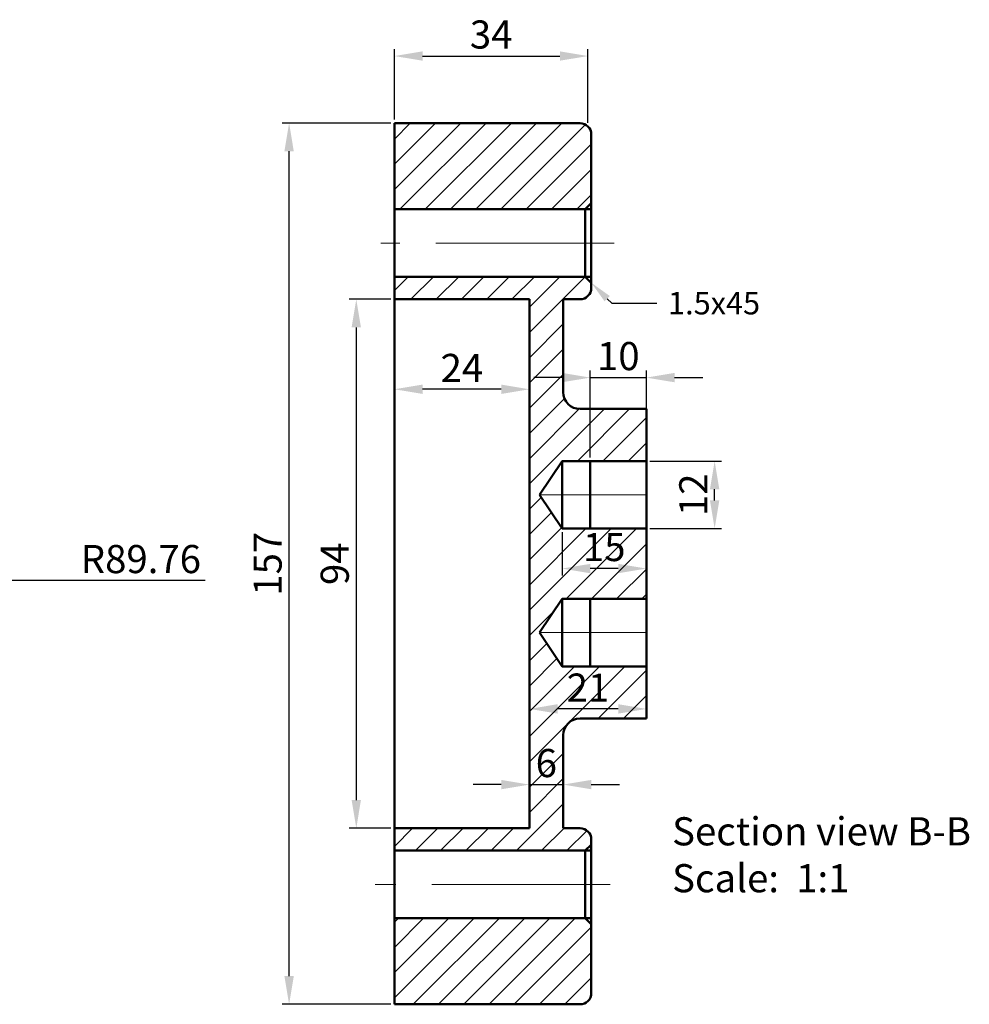
# Model space of a CAD drawing. Units: millimetres. Extents: x 2983 to 3450, y 1738 to 2029.
# Tile 3 of 3: x 3281 to 3450, y 1770 to 1945. Entities that reach past the tile are written whole.
import ezdxf
from ezdxf import colors
from ezdxf.entities.mleader import LeaderData, LeaderLine
from ezdxf.math import Vec2, Vec3

# ---------------------------------------------------------------- set-up
doc = ezdxf.new("R2010")
doc.units = ezdxf.units.MM
doc.linetypes.add('CENTER', pattern=[50.8, 31.75, -6.35, 6.35, -6.35])
for name, color, linetype, lineweight in [('M-CNTR', 1, 'CENTER', 18), ('M-DIMS', 2, 'Continuous', 25), ('M-HATC', 8, 'Continuous', 18), ('M-OUTL', 7, 'Continuous', 50), ('M-TEXT', 3, 'Continuous', 25)]:
    doc.layers.add(name, color=color, linetype=linetype, lineweight=lineweight)
doc.styles.get("Standard").update_dxf_attribs({"font": 'arial.ttf'})
doc.dimstyles.new('ISO-25', dxfattribs={"dimtxt": 5, "dimasz": 5, "dimexe": 1.25, "dimexo": 0.625, "dimtad": 1, "dimdec": 0, "dimtxsty": 'Standard', "dimcen": 2.5, "dimadec": 0, "dimazin": 0, "dimtfac": 1, "dimtdec": 0, "dimtmove": 0, "dimatfit": 3, "dimfxl": 1, "dimarcsym": 0})

# ---------------------------------------------------------------- blocks, each defined once
blk = doc.blocks.new('*D26')
at = {"layer": 'Defpoints', "color": 0, "transparency": 16777216}
for p in [(3347.39, 1895.31), (3371.39, 1895.31), (3347.39, 1879.32)]:
    blk.add_point(p, dxfattribs=at)
at = {"layer": 'M-DIMS', "color": 0, "lineweight": -2, "transparency": 16777216}
for p, q in [((3347.39, 1894.69), (3347.39, 1878.07)), ((3371.39, 1894.69), (3371.39, 1878.07)), ((3366.39, 1879.32), (3352.39, 1879.32))]:
    blk.add_line(p, q, dxfattribs=at)
at = {"layer": 'M-DIMS', "color": 0, "transparency": 16777216}
for points in [[(3352.39, 1880.15), (3352.39, 1878.49), (3347.39, 1879.32)], [(3366.39, 1880.15), (3366.39, 1878.49), (3371.39, 1879.32)]]:
    blk.add_solid(points, dxfattribs=at)
at = {"layer": 'M-DIMS', "color": 0, "transparency": 16777216, "insert": (3359.39, 1882.46), "char_height": 5, "attachment_point": 5}
blk.add_mtext('24', dxfattribs=at)
blk = doc.blocks.new('*D27')
at = {"layer": 'Defpoints', "color": 0, "transparency": 16777216}
for p in [(3381.8, 1938.55), (3347.39, 1926.63), (3381.8, 1926.04)]:
    blk.add_point(p, dxfattribs=at)
at = {"layer": 'M-DIMS', "color": 0, "lineweight": -2, "transparency": 16777216}
for p, q in [((3347.39, 1927.25), (3347.39, 1939.8)), ((3381.8, 1926.67), (3381.8, 1939.8)), ((3352.39, 1938.55), (3376.8, 1938.55))]:
    blk.add_line(p, q, dxfattribs=at)
at = {"layer": 'M-DIMS', "color": 0, "transparency": 16777216}
for points in [[(3352.39, 1939.38), (3352.39, 1937.72), (3347.39, 1938.55)], [(3376.8, 1939.38), (3376.8, 1937.72), (3381.8, 1938.55)]]:
    blk.add_solid(points, dxfattribs=at)
at = {"layer": 'M-DIMS', "color": 0, "transparency": 16777216, "insert": (3364.59, 1941.73), "char_height": 5, "attachment_point": 5}
blk.add_mtext('34', dxfattribs=at)
blk = doc.blocks.new('*D28')
at = {"layer": 'Defpoints', "color": 0, "transparency": 16777216}
for p in [(3392.19, 1881.39), (3382.19, 1866.56), (3392.19, 1866.56)]:
    blk.add_point(p, dxfattribs=at)
at = {"layer": 'M-DIMS', "color": 0, "lineweight": -2, "transparency": 16777216}
for p, q in [((3382.19, 1867.19), (3382.19, 1882.64)), ((3392.19, 1867.19), (3392.19, 1882.64)), ((3377.19, 1881.39), (3372.19, 1881.39)), ((3382.19, 1881.39), (3392.19, 1881.39)), ((3397.19, 1881.39), (3402.19, 1881.39))]:
    blk.add_line(p, q, dxfattribs=at)
at = {"layer": 'M-DIMS', "color": 0, "transparency": 16777216}
for points in [[(3377.19, 1882.23), (3377.19, 1880.56), (3382.19, 1881.39)], [(3397.19, 1882.23), (3397.19, 1880.56), (3392.19, 1881.39)]]:
    blk.add_solid(points, dxfattribs=at)
at = {"layer": 'M-DIMS', "color": 0, "transparency": 16777216, "insert": (3387.19, 1884.57), "char_height": 5, "attachment_point": 5}
blk.add_mtext('10', dxfattribs=at)
blk = doc.blocks.new('*D29')
at = {"layer": 'Defpoints', "color": 0, "transparency": 16777216}
for p in [(3371.39, 1830.06), (3392.19, 1830.06), (3371.39, 1822.5)]:
    blk.add_point(p, dxfattribs=at)
at = {"layer": 'M-DIMS', "color": 0, "lineweight": -2, "transparency": 16777216}
for p, q in [((3371.39, 1829.44), (3371.39, 1821.25)), ((3392.19, 1829.44), (3392.19, 1821.25)), ((3387.19, 1822.5), (3376.39, 1822.5))]:
    blk.add_line(p, q, dxfattribs=at)
at = {"layer": 'M-DIMS', "color": 0, "transparency": 16777216}
for points in [[(3376.39, 1823.34), (3376.39, 1821.67), (3371.39, 1822.5)], [(3387.19, 1823.34), (3387.19, 1821.67), (3392.19, 1822.5)]]:
    blk.add_solid(points, dxfattribs=at)
at = {"layer": 'M-DIMS', "color": 0, "transparency": 16777216, "insert": (3381.79, 1825.64), "char_height": 5, "attachment_point": 5}
blk.add_mtext('21', dxfattribs=at)
blk = doc.blocks.new('*D30')
at = {"layer": 'Defpoints', "color": 0, "transparency": 16777216}
for p in [(3377.19, 1854.56), (3392.19, 1854.56), (3377.19, 1847.45)]:
    blk.add_point(p, dxfattribs=at)
at = {"layer": 'M-DIMS', "color": 0, "lineweight": -2, "transparency": 16777216}
for p, q in [((3377.19, 1853.94), (3377.19, 1846.2)), ((3392.19, 1853.94), (3392.19, 1846.2)), ((3387.19, 1847.45), (3382.19, 1847.45))]:
    blk.add_line(p, q, dxfattribs=at)
at = {"layer": 'M-DIMS', "color": 0, "transparency": 16777216}
for points in [[(3382.19, 1848.28), (3382.19, 1846.62), (3377.19, 1847.45)], [(3387.19, 1848.28), (3387.19, 1846.62), (3392.19, 1847.45)]]:
    blk.add_solid(points, dxfattribs=at)
at = {"layer": 'M-DIMS', "color": 0, "transparency": 16777216, "insert": (3384.69, 1850.63), "char_height": 5, "attachment_point": 5}
blk.add_mtext('15', dxfattribs=at)
blk = doc.blocks.new('*D31')
at = {"layer": 'Defpoints', "color": 0, "transparency": 16777216}
for p in [(3392.19, 1866.56), (3404.31, 1866.56), (3392.19, 1854.56)]:
    blk.add_point(p, dxfattribs=at)
at = {"layer": 'M-DIMS', "color": 0, "lineweight": -2, "transparency": 16777216}
for p, q in [((3392.81, 1866.56), (3405.56, 1866.56)), ((3404.31, 1859.56), (3404.31, 1861.56)), ((3392.81, 1854.56), (3405.56, 1854.56))]:
    blk.add_line(p, q, dxfattribs=at)
at = {"layer": 'M-DIMS', "color": 0, "transparency": 16777216}
for points in [[(3403.48, 1861.56), (3405.14, 1861.56), (3404.31, 1866.56)], [(3403.48, 1859.56), (3405.14, 1859.56), (3404.31, 1854.56)]]:
    blk.add_solid(points, dxfattribs=at)
at = {"layer": 'M-DIMS', "color": 0, "transparency": 16777216, "insert": (3401.17, 1860.56), "char_height": 5, "attachment_point": 5, "rotation": 90}
blk.add_mtext('12', dxfattribs=at)
blk = doc.blocks.new('*D32')
at = {"layer": 'Defpoints', "color": 0, "transparency": 16777216}
for p in [(3347.39, 1895.31), (3340.62, 1801.31), (3347.39, 1801.31)]:
    blk.add_point(p, dxfattribs=at)
at = {"layer": 'M-DIMS', "color": 0, "lineweight": -2, "transparency": 16777216}
for p, q in [((3346.76, 1895.31), (3339.37, 1895.31)), ((3340.62, 1890.31), (3340.62, 1806.31)), ((3346.76, 1801.31), (3339.37, 1801.31))]:
    blk.add_line(p, q, dxfattribs=at)
at = {"layer": 'M-DIMS', "color": 0, "transparency": 16777216}
for points in [[(3339.79, 1890.31), (3341.45, 1890.31), (3340.62, 1895.31)], [(3339.79, 1806.31), (3341.45, 1806.31), (3340.62, 1801.31)]]:
    blk.add_solid(points, dxfattribs=at)
at = {"layer": 'M-DIMS', "color": 0, "transparency": 16777216, "insert": (3337.44, 1848.31), "char_height": 5, "attachment_point": 5, "rotation": 90}
blk.add_mtext('94', dxfattribs=at)
blk = doc.blocks.new('*D33')
at = {"layer": 'Defpoints', "color": 0, "transparency": 16777216}
for p in [(3328.68, 1926.63), (3347.39, 1926.63), (3347.39, 1770)]:
    blk.add_point(p, dxfattribs=at)
at = {"layer": 'M-DIMS', "color": 0, "lineweight": -2, "transparency": 16777216}
for p, q in [((3346.76, 1926.63), (3327.43, 1926.63)), ((3328.68, 1775), (3328.68, 1921.63)), ((3346.76, 1770), (3327.43, 1770))]:
    blk.add_line(p, q, dxfattribs=at)
at = {"layer": 'M-DIMS', "color": 0, "transparency": 16777216}
for points in [[(3327.84, 1921.63), (3329.51, 1921.63), (3328.68, 1926.63)], [(3327.84, 1775), (3329.51, 1775), (3328.68, 1770)]]:
    blk.add_solid(points, dxfattribs=at)
at = {"layer": 'M-DIMS', "color": 0, "transparency": 16777216, "insert": (3325.5, 1848.31), "char_height": 5, "attachment_point": 5, "rotation": 90}
blk.add_mtext('157', dxfattribs=at)
blk = doc.blocks.new('*D34')
at = {"layer": 'Defpoints', "color": 0, "transparency": 16777216}
for p in [(3377.39, 1809.05), (3371.39, 1801.31), (3377.39, 1801.31)]:
    blk.add_point(p, dxfattribs=at)
at = {"layer": 'M-DIMS', "color": 0, "lineweight": -2, "transparency": 16777216}
for p, q in [((3371.39, 1801.94), (3371.39, 1810.3)), ((3377.39, 1801.94), (3377.39, 1810.3)), ((3366.39, 1809.05), (3361.39, 1809.05)), ((3371.39, 1809.05), (3377.39, 1809.05)), ((3382.39, 1809.05), (3387.39, 1809.05))]:
    blk.add_line(p, q, dxfattribs=at)
at = {"layer": 'M-DIMS', "color": 0, "transparency": 16777216}
for points in [[(3366.39, 1809.88), (3366.39, 1808.22), (3371.39, 1809.05)], [(3382.39, 1809.88), (3382.39, 1808.22), (3377.39, 1809.05)]]:
    blk.add_solid(points, dxfattribs=at)
at = {"layer": 'M-DIMS', "color": 0, "transparency": 16777216, "insert": (3374.39, 1812.23), "char_height": 5, "attachment_point": 5}
blk.add_mtext('6', dxfattribs=at)
blk = doc.blocks.new('*D43')
at = {"layer": 'Defpoints', "color": 0, "transparency": 16777216}
for p in [(3158.71, 1845.31), (3248.47, 1845.31)]:
    blk.add_point(p, dxfattribs=at)
at = {"layer": 'M-DIMS', "color": 0, "lineweight": -2, "transparency": 16777216}
for p, q in [((3158.71, 1845.31), (3248.47, 1845.31)), ((3313.78, 1845.31), (3253.47, 1845.31))]:
    blk.add_line(p, q, dxfattribs=at)
at = {"layer": 'M-DIMS', "color": 0, "transparency": 16777216}
blk.add_solid([(3253.47, 1846.15), (3253.47, 1844.48), (3248.47, 1845.31)], dxfattribs=at)
at = {"layer": 'M-DIMS', "color": 0, "transparency": 16777216, "insert": (3302.33, 1848.49), "char_height": 5, "attachment_point": 5, "rotation": 0.0003}
blk.add_mtext('R89.76', dxfattribs=at)

msp = doc.modelspace()

# ---------------------------------------------------------------- hatches: boundary and pattern name
at = {"layer": 'M-HATC'}
h = msp.add_hatch(dxfattribs=at)
h.set_pattern_fill('ANSI31', color=256)
h.set_pattern_definition([(45, (-31.2105, 0), (-2.245064, 2.245064), [])])
h.paths.add_polyline_path([(3347.386, 1926.627), (3347.386, 1911.312), (3381.326, 1911.312), (3382.386, 1912.372), (3382.386, 1924.627, 0.4142136), (3380.386, 1926.627)])
h.paths.add_polyline_path([(3347.386, 1899.312), (3347.386, 1895.312), (3371.386, 1895.312), (3371.386, 1848.312), (3371.386, 1801.312), (3347.386, 1801.312), (3347.386, 1797.312), (3381.326, 1797.312), (3382.386, 1798.372), (3382.386, 1799.312, 0.4142136), (3380.386, 1801.312), (3377.386, 1801.312), (3377.386, 1817.812, -0.4142136), (3380.386, 1820.812), (3382.185, 1820.812), (3392.185, 1820.812), (3392.185, 1830.062), (3382.185, 1830.062), (3377.185, 1830.062), (3373.185, 1836.062), (3377.185, 1842.062), (3382.185, 1842.062), (3392.185, 1842.062), (3392.185, 1848.312), (3392.185, 1854.562), (3382.185, 1854.562), (3377.185, 1854.562), (3373.185, 1860.562), (3377.185, 1866.562), (3382.185, 1866.562), (3392.185, 1866.562), (3392.185, 1875.812), (3382.185, 1875.812), (3380.386, 1875.812, -0.4142136), (3377.386, 1878.812), (3377.386, 1895.312), (3380.386, 1895.312, 0.4142136), (3382.386, 1897.312), (3382.386, 1898.251), (3381.326, 1899.312)])
h.paths.add_polyline_path([(3347.386, 1785.312), (3347.386, 1769.996), (3380.386, 1769.996, 0.4142136), (3382.386, 1771.996), (3382.386, 1784.251), (3381.326, 1785.312)])

# ---------------------------------------------------------------- linework, layer by layer
at = {"layer": 'M-CNTR'}
for p, q in [((3386.481, 1905.312), (3344.985, 1905.312)), ((3373.185, 1860.562), (3392.185, 1860.562)), ((3373.185, 1836.062), (3392.185, 1836.062)), ((3385.771, 1791.312), (3343.999, 1791.312))]:
    msp.add_line(p, q, dxfattribs=at)
at = {"layer": 'M-OUTL'}
for p, q in [((3347.386, 1848.312), (3347.386, 1926.627)), ((3347.386, 1926.627), (3380.386, 1926.627)), ((3382.386, 1924.627), (3382.386, 1897.312)), ((3382.386, 1911.312), (3347.386, 1911.312)), ((3381.326, 1911.312), (3382.386, 1912.372)), ((3381.326, 1911.312), (3381.326, 1899.312)), ((3382.386, 1899.312), (3347.386, 1899.312)), ((3381.326, 1899.312), (3382.386, 1898.251)), ((3347.386, 1895.312), (3371.386, 1895.312)), ((3371.386, 1895.312), (3371.386, 1848.312)), ((3380.386, 1895.312), (3377.386, 1895.312)), ((3377.386, 1895.312), (3377.386, 1878.812)), ((3380.386, 1875.812), (3382.185, 1875.812)), ((3382.185, 1875.812), (3392.185, 1875.812)), ((3392.185, 1875.812), (3392.185, 1854.562)), ((3377.185, 1866.562), (3373.185, 1860.562)), ((3377.185, 1854.562), (3377.185, 1866.562)), ((3377.185, 1866.562), (3382.185, 1866.562)), ((3382.185, 1854.562), (3382.185, 1866.562)), ((3382.185, 1866.562), (3392.185, 1866.562)), ((3373.185, 1860.562), (3377.185, 1854.562)), ((3382.185, 1854.562), (3377.185, 1854.562)), ((3392.185, 1854.562), (3382.185, 1854.562)), ((3392.185, 1848.312), (3392.185, 1854.562)), ((3347.386, 1848.312), (3347.386, 1769.996)), ((3371.386, 1801.312), (3371.386, 1848.312)), ((3392.185, 1848.312), (3392.185, 1842.062)), ((3373.185, 1836.062), (3377.185, 1842.062)), ((3382.185, 1842.062), (3377.185, 1842.062)), ((3377.185, 1842.062), (3377.185, 1830.062)), ((3392.185, 1842.062), (3382.185, 1842.062)), ((3382.185, 1842.062), (3382.185, 1830.062)), ((3392.185, 1820.812), (3392.185, 1842.062)), ((3377.185, 1830.062), (3373.185, 1836.062)), ((3377.185, 1830.062), (3382.185, 1830.062)), ((3382.185, 1830.062), (3392.185, 1830.062)), ((3380.386, 1820.812), (3382.185, 1820.812)), ((3382.185, 1820.812), (3392.185, 1820.812)), ((3377.386, 1801.312), (3377.386, 1817.812)), ((3347.386, 1801.312), (3371.386, 1801.312)), ((3380.386, 1801.312), (3377.386, 1801.312)), ((3382.386, 1771.996), (3382.386, 1799.312)), ((3381.326, 1797.312), (3382.386, 1798.372)), ((3382.386, 1797.312), (3347.386, 1797.312)), ((3381.326, 1785.312), (3381.326, 1797.312)), ((3382.386, 1785.312), (3347.386, 1785.312)), ((3381.326, 1785.312), (3382.386, 1784.251)), ((3347.386, 1769.996), (3380.386, 1769.996))]:
    msp.add_line(p, q, dxfattribs=at)
for centre, radius, start, end in [((3380.386, 1924.627), 2, 0, 90), ((3380.386, 1897.312), 2, 270, 0), ((3380.386, 1878.812), 3, 180, 270), ((3380.386, 1817.812), 3, 90, 180), ((3380.386, 1799.312), 2, 0, 90), ((3380.386, 1771.996), 2, 270, 0)]:
    msp.add_arc(centre, radius, start, end, dxfattribs=at)

# ---------------------------------------------------------------- texts
at = {"layer": 'M-TEXT', "insert": (3396.752, 1803.245), "char_height": 5, "attachment_point": 1}
msp.add_mtext_dynamic_manual_height_columns('Section view B-B\\PScale:  1:1', width=86.4063, gutter_width=12.5, heights=[0], dxfattribs=at)

# ---------------------------------------------------------------- dimensions: what is measured, and where the dimension line sits
at = {"layer": 'M-DIMS'}
for base, p1, p2, picture, middle in [((3381.801, 1938.551), (3347.386, 1926.627), (3381.801, 1926.042), '*D27', (3364.594, 1941.73)), ((3347.386, 1879.321), (3371.386, 1895.312), (3347.386, 1895.312), '*D26', (3359.386, 1882.456)), ((3392.185, 1881.395), (3382.185, 1866.562), (3392.185, 1866.562), '*D28', (3387.185, 1884.573)), ((3377.185, 1847.449), (3392.185, 1854.562), (3377.185, 1854.562), '*D30', (3384.685, 1850.627)), ((3371.386, 1822.504), (3392.185, 1830.062), (3371.386, 1830.062), '*D29', (3381.786, 1825.639)), ((3377.386, 1809.05), (3371.386, 1801.312), (3377.386, 1801.312), '*D34', (3374.386, 1812.228))]:
    dim = msp.add_linear_dim(base=base, p1=p1, p2=p2, dimstyle='ISO-25', override={"dimclrd": 0, "dimclre": 0, "dimclrt": 0}, dxfattribs=at)
    dim.commit()
    dim.dimension.update_dxf_attribs({"geometry": picture, "text_midpoint": middle})
for base, p1, p2, picture, middle in [((3328.677, 1926.627), (3347.386, 1769.996), (3347.386, 1926.627), '*D33', (3325.499, 1848.312)), ((3340.621, 1801.312), (3347.386, 1895.312), (3347.386, 1801.312), '*D32', (3337.443, 1848.312)), ((3404.309, 1866.562), (3392.185, 1854.562), (3392.185, 1866.562), '*D31', (3401.174, 1860.562))]:
    dim = msp.add_linear_dim(base=base, p1=p1, p2=p2, angle=90, dimstyle='ISO-25', override={"dimclrd": 0, "dimclre": 0, "dimclrt": 0}, dxfattribs=at)
    dim.commit()
    dim.dimension.update_dxf_attribs({"geometry": picture, "text_midpoint": middle})
dim = msp.add_radius_dim(center=(3158.714, 1845.312), mpoint=(3248.475, 1845.312), dimstyle='ISO-25', override={"dimdec": 2, "dimlfac": 1, "dimrnd": 0, "dimzin": 0, "dimdsep": 46, "dimlunit": 2}, dxfattribs=at)
dim.commit()
dim.dimension.update_dxf_attribs({"geometry": '*D43', "text_midpoint": (3302.331, 1845.312), "dimtype": 164})

# ---------------------------------------------------------------- leaders
ml = msp.add_multileader_mtext('Standard', dxfattribs=at)
ml.set_content('1.5x45', color=256)
ml.set_leader_properties()
ml.build(insert=Vec2(0, 0))
ctx = ml.context
ctx.base_point, ctx.plane_origin = Vec3(3394.039, 1894.599), Vec3(3382.386, 1898.251)
notes = []
notes.append((ctx, [(0, (1, 1, 0), (3386.039, 1894.599), (1, 0), 8, [(0, [(3382.386, 1898.251)], 0, [])])]))
ctx.mtext.insert, ctx.mtext.flow_direction = Vec3(3396.039, 1896.633), 5
for ctx, leaders in notes:
    for number, flags, end, landing, length, lines in leaders:
        leader = LeaderData()
        leader.index, (leader.has_last_leader_line, leader.has_dogleg_vector, leader.attachment_direction) = number, flags
        leader.last_leader_point, leader.dogleg_vector, leader.dogleg_length = Vec3(end), Vec3(landing), length
        for number, points, colour, breaks in lines:
            line = LeaderLine()
            line.index, line.vertices, line.color, line.breaks = number, Vec3.list(points), colors.encode_raw_color(colour), breaks
            leader.lines.append(line)
        ctx.leaders.append(leader)

doc.saveas('drawing.dxf')
